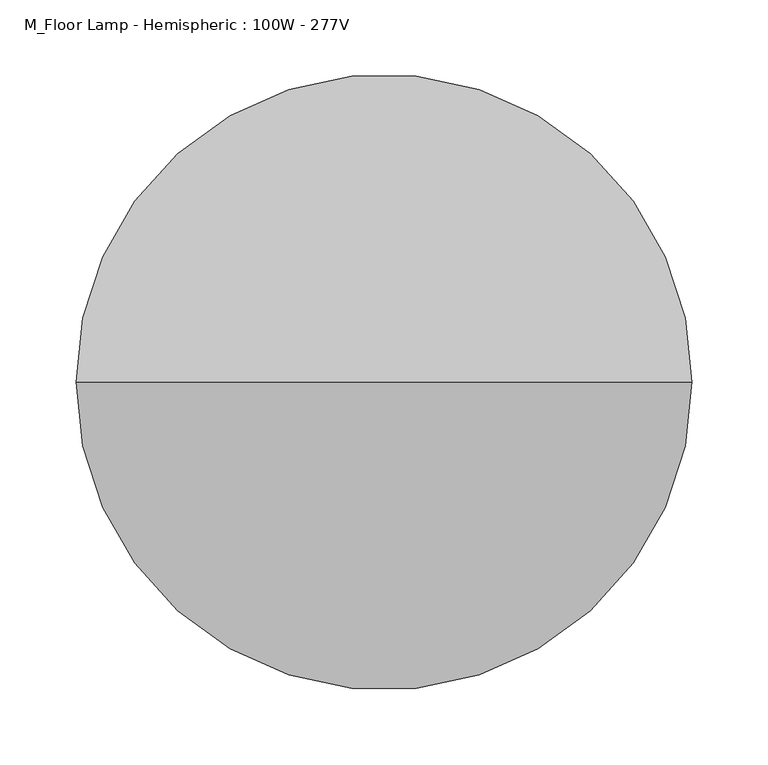
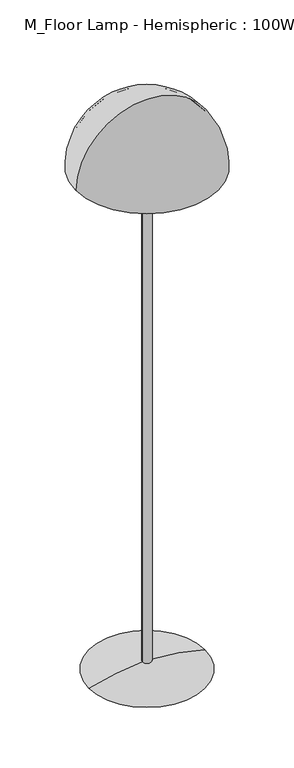
"""IFC4 building model written with IfcOpenShell, lengths in millimetres: light fixture geometry, M_Floor Lamp - Hemispheric : 100W - 277V."""

from ifc_helpers import new_model, si_unit, point, frame, origin, origin_with_axes, origin_2d, place, context, project, spatial, polyline, circle_curve, ellipse_curve, trimmed, segment, composite_curve, outline, extrude, source, transform, mapped, element, save
from ifc_brep_helpers import plane_surface, revolved_surface, advanced_brep


def m_floor_lamp_hemispheric_100w_277v_4a08ccbb(model_context):
    return source(origin(), model_context, "Body", "SolidModel", [
        extrude(outline(composite_curve([segment(trimmed(circle_curve(origin_2d(), 12.7), [point((-12.7, 0.0))], [point((12.7, 0.0))], False, "CARTESIAN"), True, "CONTINUOUS"), segment(trimmed(circle_curve(origin_2d(), 12.7), [point((12.7, 0.0))], [point((-12.7, 0.0))], False, "CARTESIAN"), True, "CONTINUOUS")], self_intersect=False)), frame((0.0, 0.0, 25.4), z_axis=(0.0, 0.0, 1.0), x_axis=(1.0, 0.0, 0.0)), (0.0, 0.0, 1.0), 1524.0),
        advanced_brep(
        [(-165.1, 0.0, 0.0), (165.1, 0.0, 0.0), (12.7, 0.0, 0.0), (-12.7, 0.0, 0.0), (-12.7, 0.0, 25.4), (12.7, 0.0, 25.4)],
        [
            (0, 1, circle_curve(frame((0.0, 0.0, 0.0), z_axis=(0.0, 0.0, -1.0), x_axis=(1.0, 0.0, 0.0)), 165.1)),
            (1, 2),
            (2, 3, circle_curve(origin_with_axes(), 12.7)),
            (3, 0),
            (1, 0, circle_curve(frame((0.0, 0.0, 0.0), z_axis=(0.0, 0.0, -1.0), x_axis=(1.0, 0.0, 0.0)), 165.1)),
            (3, 2, circle_curve(origin_with_axes(), 12.7)),
            (4, 5, circle_curve(frame((0.0, 0.0, 25.4), z_axis=(0.0, 0.0, -1.0), x_axis=(1.0, 0.0, 0.0)), 12.7)),
            (5, 1, circle_curve(frame((-10.5405788, 0.0, -583.9434729), z_axis=(0.0, 1.0, 0.0), x_axis=(1.0, 0.0, 0.0)), 609.7865138)),
            (0, 4, circle_curve(frame((10.5405788, 0.0, -583.9434729), z_axis=(0.0, 1.0, 0.0), x_axis=(-1.0, 0.0, 0.0)), 609.7865138)),
            (5, 4, circle_curve(frame((0.0, 0.0, 25.4), z_axis=(0.0, 0.0, -1.0), x_axis=(1.0, 0.0, 0.0)), 12.7)),
            (2, 5),
            (4, 3),
        ],
        [
            plane_surface(frame((0.0, 0.0, 0.0), z_axis=(0.0, 0.0, -1.0), x_axis=(1.0, 0.0, 0.0))),
            revolved_surface(trimmed(ellipse_curve(frame((-10.5405788, 0.0, -583.9434729), z_axis=(0.0, -1.0, 0.0), x_axis=(1.0, 0.0, 0.0)), 609.7865138, 609.7865138), [point((165.1, 0.0, 0.0))], [point((12.7, 0.0, 25.4))], True, "CARTESIAN"), (0.0, 0.0, 127.0), (0.0, 0.0, 1.0)),
            revolved_surface(polyline([(12.7, 0.0, 25.400000000000006), (12.7, 0.0, 0.0)]), (0.0, 0.0, 127.0), (0.0, 0.0, 1.0)),
        ],
        [
            (0, [[1, 2, 3, 4]]),
            (0, [[5, -4, 6, -2]]),
            (1, [[7, 8, -1, 9]]),
            (1, [[10, -9, -5, -8]]),
            (2, [[-3, 11, -7, 12]]),
            (2, [[-6, -12, -10, -11]]),
        ],
    ),
        advanced_brep(
        [(-197.591573, 0.0, 1510.4133868), (197.591573, 0.0, 1510.4133868), (0.0, 0.0, 1707.4075084), (-202.3305676, 0.0, 1510.4133868), (202.3305676, 0.0, 1510.4133868), (0.0, 0.0, 1713.4837615)],
        [
            (0, 1, circle_curve(frame((0.0, 0.0, 1510.4133868), z_axis=(0.0, 0.0, -1.0), x_axis=(1.0, 0.0, 0.0)), 197.591573)),
            (1, 2, circle_curve(frame((0.7416268, 0.0, 1510.5589055), z_axis=(0.0, -1.0, 0.0), x_axis=(1.0, 0.0, 0.0)), 196.85)),
            (2, 0, circle_curve(frame((-0.7416268, 0.0, 1510.5589055), z_axis=(0.0, -1.0, 0.0), x_axis=(-1.0, 0.0, 0.0)), 196.85)),
            (1, 0, circle_curve(frame((0.0, 0.0, 1510.4133868), z_axis=(0.0, 0.0, -1.0), x_axis=(1.0, 0.0, 0.0)), 197.591573)),
            (3, 4, circle_curve(frame((0.0, 0.0, 1510.4133868), z_axis=(0.0, 0.0, -1.0), x_axis=(1.0, 0.0, 0.0)), 202.3305676)),
            (4, 1),
            (0, 3),
            (4, 3, circle_curve(frame((0.0, 0.0, 1510.4133868), z_axis=(0.0, 0.0, -1.0), x_axis=(1.0, 0.0, 0.0)), 202.3305676)),
            (5, 4, circle_curve(frame((-0.8693923, 0.0, 1510.2856214), z_axis=(0.0, 1.0, 0.0), x_axis=(1.0, 0.0, 0.0)), 203.2)),
            (3, 5, circle_curve(frame((0.8693923, 0.0, 1510.2856214), z_axis=(0.0, 1.0, 0.0), x_axis=(-1.0, 0.0, 0.0)), 203.2)),
        ],
        [
            revolved_surface(trimmed(ellipse_curve(frame((0.7416268, 0.0, 1510.5589055), z_axis=(0.0, 1.0, 0.0), x_axis=(1.0, 0.0, 0.0)), 196.85, 196.85), [point((0.0, 0.0, 1707.4075084))], [point((197.591573, 0.0, 1510.4133868))], True, "CARTESIAN"), (0.0, 0.0, 1815.2133868), (0.0, 0.0, 1.0)),
            plane_surface(frame((0.0, 0.0, 1510.4133868), z_axis=(0.0, 0.0, -1.0), x_axis=(1.0, 0.0, 0.0))),
            revolved_surface(trimmed(ellipse_curve(frame((-0.8693923, 0.0, 1510.2856214), z_axis=(0.0, -1.0, 0.0), x_axis=(1.0, 0.0, 0.0)), 203.2, 203.2), [point((202.3305676, 0.0, 1510.4133868))], [point((0.0, 0.0, 1713.4837615))], True, "CARTESIAN"), (0.0, 0.0, 1815.2133868), (0.0, 0.0, 1.0)),
        ],
        [
            (0, [[1, 2, 3]]),
            (0, [[4, -3, -2]]),
            (1, [[5, 6, -1, 7]]),
            (1, [[8, -7, -4, -6]]),
            (2, [[9, -5, 10]]),
            (2, [[-10, -8, -9]]),
        ],
    ),
    ])


if __name__ == "__main__":
    model = new_model("IFC4")
    model_context = context("Model", 3, world=origin())
    ifc_project = project(units=[si_unit("LENGTHUNIT", "METRE", prefix="MILLI")], contexts=[model_context])
    site = spatial("IfcSite", under=ifc_project)
    building = spatial("IfcBuilding", under=site)
    placement = place(None, origin())
    m_floor_lamp_hemispheric_100w_277v_shape = m_floor_lamp_hemispheric_100w_277v_4a08ccbb(model_context)
    element("IfcLightFixture", 1, ObjectType="M_Floor Lamp - Hemispheric : 100W - 277V", at=placement, inside=building, context=model_context, shape_type="MappedRepresentation", body=[
        mapped(m_floor_lamp_hemispheric_100w_277v_shape, transform((0.0, 0.0, 0.0), x_axis=(1.0, 0.0, 0.0), y_axis=(0.0, 1.0, 0.0), z_axis=(0.0, 0.0, 1.0))),
    ])
    save(model, "model.ifc")

# Revit data of these elements
# Type "M_Floor Lamp - Hemispheric : 100W - 277V"
#   Photometric Web File = "FLH1A19.IES"
#   Assembly Code = "D5020220"
#   Lamp = "A-19"
#   Wattage Comments = "100"
#   Wattage = 100 W
#   built-in parameter 1150110 = 1 (stored number, unit not read)
#   built-in parameter 1114217 = 1 (stored number, unit not read)
#   built-in parameter 1150109 = 1 (stored number, unit not read)
#   built-in parameter 1150113 = 1 (stored number, unit not read)
#   Tilt Angle = 90.00°
#   built-in parameter 1150115 = 1 (stored number, unit not read)
#   built-in parameter 1150105 = 139.261 (stored number, unit not read)
#   built-in parameter 1150112 = 1 (stored number, unit not read)
#   built-in parameter 1150114 = 1 (stored number, unit not read)
#   built-in parameter 1150107 = 2800 (stored number, unit not read)
#   built-in parameter 1150106 = 1.39261 (stored number, unit not read)
#   built-in parameter 1150104 = 1.6258 (stored number, unit not read)
#   Voltage = 277 V
#   built-in parameter 1114218 = 1 (stored number, unit not read)
#   built-in parameter 1150133 = 10 (stored number, unit not read)
#   Lumens = 1750 lm
#   Apparent Load = 100 VA
#   built-in parameter 1150134 = 4
#   built-in parameter 1150137 = 1
#   Color Filter = 16777215
#   Number of poles = 1
#   Shade Material = Plastic, Lamp Shade
#   Stand Material = Steel, Chrome Plated
#   Dimming Lamp Color Temperature Shift = (empty or 0)
#   Default Elevation = 0
# Element 1 (IfcLightFixture, "M_Floor Lamp - Hemispheric : 100W - 277V")
#   Materials on its faces: "Steel, Chrome Plated", "Plastic, Lamp Shade"
# Materials
#   "Plastic, Lamp Shade": class "Glass", colour RGB 250 244 225, transparency 0.58, Description = "physical material", Cost = 0
#   "Steel, Chrome Plated": class "Metal", colour RGB 17 17 17, transparency 0, Description = "Chromiuim plated steel", Cost = 0
